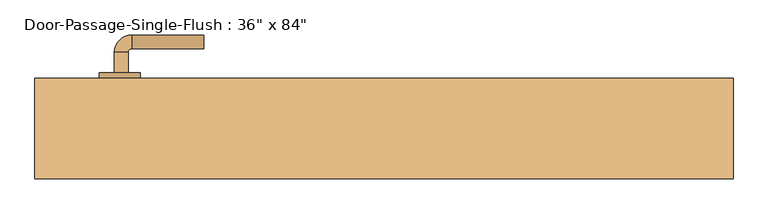
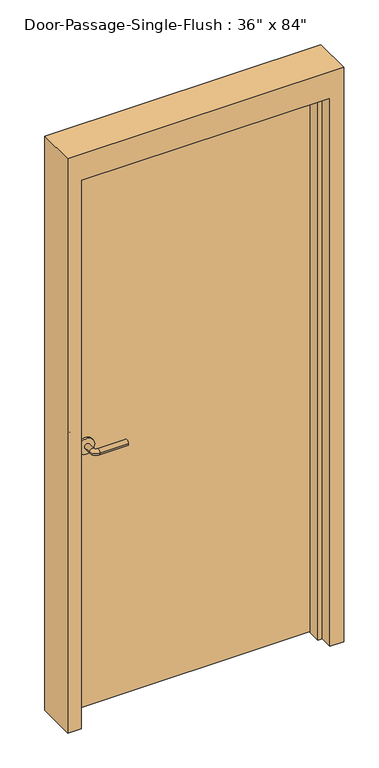
"""IFC4 building model written with IfcOpenShell, lengths in millimetres: door geometry."""

from ifc_helpers import new_model, si_unit, point, frame, frame_2d, origin, origin_with_axes, place, context, project, spatial, polyline, circle_curve, ellipse_curve, trimmed, segment, composite_curve, outline, extrude, faceted_brep, source, transform, mapped, element, save
from ifc_brep_helpers import plane_surface, cylinder_surface, revolved_surface, advanced_brep


def door_9ff278b0(model_context):
    return source(origin(), model_context, "Body", "SolidModel", [
        advanced_brep(
        [(-392.190625, 42.8, 1016.0), (-372.190625, 42.8, 1016.0), (-372.190625, 12.8, 1016.0), (-392.190625, 12.8, 1016.0), (-367.190625, 7.8, 1016.0), (-367.190625, -12.2, 1016.0), (-262.190625, -12.2, 1016.0), (-262.190625, 7.8, 1016.0)],
        [
            (0, 1, circle_curve(frame((-382.190625, 42.8, 1016.0), z_axis=(0.0, 1.0, 0.0), x_axis=(1.0, 0.0, 0.0)), 10.0)),
            (1, 0, circle_curve(frame((-382.190625, 42.8, 1016.0), z_axis=(0.0, 1.0, 0.0), x_axis=(1.0, 0.0, 0.0)), 10.0)),
            (1, 2),
            (2, 3, circle_curve(frame((-382.190625, 12.8, 1016.0), z_axis=(0.0, 1.0, 0.0), x_axis=(1.0, 0.0, 0.0)), 10.0)),
            (3, 0),
            (3, 2, circle_curve(frame((-382.190625, 12.8, 1016.0), z_axis=(0.0, 1.0, 0.0), x_axis=(1.0, 0.0, 0.0)), 10.0)),
            (4, 5, circle_curve(frame((-367.190625, -2.2, 1016.0), z_axis=(-1.0, 0.0, 0.0), x_axis=(0.0, 1.0, 0.0)), 10.0)),
            (5, 3, circle_curve(frame((-367.190625, 12.8, 1016.0), z_axis=(0.0, 0.0, -1.0), x_axis=(-1.0, 0.0, 0.0)), 25.0)),
            (2, 4, circle_curve(frame((-367.190625, 12.8, 1016.0), z_axis=(0.0, 0.0, 1.0), x_axis=(-1.0, 0.0, 0.0)), 5.0)),
            (5, 4, circle_curve(frame((-367.190625, -2.2, 1016.0), z_axis=(-1.0, 0.0, 0.0), x_axis=(0.0, 1.0, 0.0)), 10.0)),
            (6, 7, circle_curve(frame((-262.190625, -2.2, 1016.0), z_axis=(1.0, 0.0, 0.0), x_axis=(0.0, 1.0, 0.0)), 10.0)),
            (7, 6, circle_curve(frame((-262.190625, -2.2, 1016.0), z_axis=(1.0, 0.0, 0.0), x_axis=(0.0, 1.0, 0.0)), 10.0)),
            (4, 7),
            (6, 5),
        ],
        [
            plane_surface(frame((-382.190625, 42.8, 1016.0), z_axis=(0.0, 1.0, 0.0), x_axis=(0.0, 0.0, 1.0))),
            cylinder_surface(frame((-382.190625, 42.8, 1016.0), z_axis=(0.0, 1.0, 0.0), x_axis=(1.0, 0.0, 0.0)), 10.0),
            revolved_surface(trimmed(ellipse_curve(frame((-382.190625, 12.8, 1016.0), z_axis=(0.0, -1.0, 0.0), x_axis=(1.0, 0.0, 0.0)), 10.0, 10.0), [point((-392.190625, 12.8, 1016.0))], [point((-372.190625, 12.8, 1016.0))], True, "CARTESIAN"), (-367.190625, 12.8, 1016.0), (0.0, 0.0, -1.0)),
            revolved_surface(trimmed(ellipse_curve(frame((-382.190625, 12.8, 1016.0), z_axis=(0.0, -1.0, 0.0), x_axis=(1.0, 0.0, 0.0)), 10.0, 10.0), [point((-372.190625, 12.8, 1016.0))], [point((-392.190625, 12.8, 1016.0))], True, "CARTESIAN"), (-367.190625, 12.8, 1016.0), (0.0, 0.0, -1.0)),
            plane_surface(frame((-262.190625, -2.2, 1016.0), z_axis=(1.0, 0.0, 0.0), x_axis=(0.0, 0.0, 1.0))),
            cylinder_surface(frame((-367.190625, -2.2, 1016.0), z_axis=(-1.0, 0.0, 0.0), x_axis=(0.0, 1.0, 0.0)), 10.0),
        ],
        [
            (0, [[1, 2]]),
            (1, [[3, 4, 5, -2]]),
            (1, [[-5, 6, -3, -1]]),
            (2, [[7, 8, -4, 9]]),
            (3, [[10, -9, -6, -8]]),
            (4, [[11, 12]]),
            (5, [[13, -11, 14, -7]]),
            (5, [[-14, -12, -13, -10]]),
        ],
    ),
        extrude(outline(composite_curve([segment(trimmed(circle_curve(frame_2d((1016.0, -384.690625)), 30.0), [point((1016.0, -414.690625))], [point((1016.0, -354.690625))], False, "CARTESIAN"), True, "CONTINUOUS"), segment(trimmed(circle_curve(frame_2d((1016.0, -384.690625)), 30.0), [point((1016.0, -354.690625))], [point((1016.0, -414.690625))], False, "CARTESIAN"), True, "CONTINUOUS")], self_intersect=False)), frame((0.0, 42.8, 0.0), z_axis=(0.0, 1.0, 0.0), x_axis=(0.0, 0.0, 1.0)), (0.0, 0.0, 1.0), 8.0),
        advanced_brep(
        [(-392.190625, 103.25, 1016.0), (-372.190625, 103.25, 1016.0), (-392.190625, 133.25, 1016.0), (-372.190625, 133.25, 1016.0), (-367.190625, 138.25, 1016.0), (-367.190625, 158.25, 1016.0), (-262.190625, 158.25, 1016.0), (-262.190625, 138.25, 1016.0)],
        [
            (0, 1, circle_curve(frame((-382.190625, 103.25, 1016.0), z_axis=(0.0, -1.0, 0.0), x_axis=(1.0, 0.0, 0.0)), 10.0)),
            (1, 0, circle_curve(frame((-382.190625, 103.25, 1016.0), z_axis=(0.0, -1.0, 0.0), x_axis=(1.0, 0.0, 0.0)), 10.0)),
            (0, 2),
            (2, 3, circle_curve(frame((-382.190625, 133.25, 1016.0), z_axis=(0.0, -1.0, 0.0), x_axis=(1.0, 0.0, 0.0)), 10.0)),
            (3, 1),
            (3, 2, circle_curve(frame((-382.190625, 133.25, 1016.0), z_axis=(0.0, -1.0, 0.0), x_axis=(1.0, 0.0, 0.0)), 10.0)),
            (4, 3, circle_curve(frame((-367.190625, 133.25, 1016.0), z_axis=(0.0, 0.0, 1.0), x_axis=(-1.0, 0.0, 0.0)), 5.0)),
            (2, 5, circle_curve(frame((-367.190625, 133.25, 1016.0), z_axis=(0.0, 0.0, -1.0), x_axis=(-1.0, 0.0, 0.0)), 25.0)),
            (5, 4, circle_curve(frame((-367.190625, 148.25, 1016.0), z_axis=(-1.0, 0.0, 0.0), x_axis=(0.0, -1.0, 0.0)), 10.0)),
            (4, 5, circle_curve(frame((-367.190625, 148.25, 1016.0), z_axis=(-1.0, 0.0, 0.0), x_axis=(0.0, -1.0, 0.0)), 10.0)),
            (6, 7, circle_curve(frame((-262.190625, 148.25, 1016.0), z_axis=(1.0, 0.0, 0.0), x_axis=(0.0, -1.0, 0.0)), 10.0)),
            (7, 6, circle_curve(frame((-262.190625, 148.25, 1016.0), z_axis=(1.0, 0.0, 0.0), x_axis=(0.0, -1.0, 0.0)), 10.0)),
            (5, 6),
            (7, 4),
        ],
        [
            plane_surface(frame((-382.190625, 103.25, 1016.0), z_axis=(0.0, -1.0, 0.0), x_axis=(0.0, 0.0, 1.0))),
            cylinder_surface(frame((-382.190625, 103.25, 1016.0), z_axis=(0.0, -1.0, 0.0), x_axis=(1.0, 0.0, 0.0)), 10.0),
            revolved_surface(trimmed(ellipse_curve(frame((-382.190625, 133.25, 1016.0), z_axis=(0.0, -1.0, 0.0), x_axis=(1.0, 0.0, 0.0)), 10.0, 10.0), [point((-392.190625, 133.25, 1016.0))], [point((-372.190625, 133.25, 1016.0))], True, "CARTESIAN"), (-367.190625, 133.25, 1016.0), (0.0, 0.0, -1.0)),
            revolved_surface(trimmed(ellipse_curve(frame((-382.190625, 133.25, 1016.0), z_axis=(0.0, -1.0, 0.0), x_axis=(1.0, 0.0, 0.0)), 10.0, 10.0), [point((-372.190625, 133.25, 1016.0))], [point((-392.190625, 133.25, 1016.0))], True, "CARTESIAN"), (-367.190625, 133.25, 1016.0), (0.0, 0.0, -1.0)),
            plane_surface(frame((-262.190625, 148.25, 1016.0), z_axis=(1.0, 0.0, 0.0), x_axis=(0.0, 0.0, 1.0))),
            cylinder_surface(frame((-367.190625, 148.25, 1016.0), z_axis=(-1.0, 0.0, 0.0), x_axis=(0.0, -1.0, 0.0)), 10.0),
        ],
        [
            (0, [[1, 2]]),
            (1, [[-1, 3, 4, 5]]),
            (1, [[-2, -5, 6, -3]]),
            (2, [[7, -4, 8, 9]]),
            (3, [[-8, -6, -7, 10]]),
            (4, [[11, 12]]),
            (5, [[-9, 13, -12, 14]]),
            (5, [[-10, -14, -11, -13]]),
        ],
    ),
        extrude(outline(composite_curve([segment(trimmed(circle_curve(frame_2d((1016.0, -384.690625)), 30.0), [point((1016.0, -414.690625))], [point((1016.0, -354.690625))], False, "CARTESIAN"), True, "CONTINUOUS"), segment(trimmed(circle_curve(frame_2d((1016.0, -384.690625)), 30.0), [point((1016.0, -354.690625))], [point((1016.0, -414.690625))], False, "CARTESIAN"), True, "CONTINUOUS")], self_intersect=False)), frame((0.0, 95.25, 0.0), z_axis=(0.0, 1.0, 0.0), x_axis=(0.0, 0.0, 1.0)), (0.0, 0.0, 1.0), 8.0),
        faceted_brep([(457.2, 46.0375, 0.0), (457.2, 95.25, 0.0), (508.0, 95.25, 0.0), (508.0, -50.8, 0.0), (457.2, -50.8, 0.0), (457.2, -1.5875, 0.0), (441.325, -1.5875, 0.0), (441.325, 46.0375, 0.0), (457.2, 46.0375, 2133.6), (457.2, 95.25, 2133.6), (-457.2, 95.25, 2133.6), (-457.2, 95.25, 0.0), (-508.0, 95.25, 0.0), (-508.0, 95.25, 2235.2), (508.0, 95.25, 2235.2), (508.0, -50.8, 2235.2), (-508.0, -50.8, 2235.2), (-508.0, -50.8, 0.0), (-457.2, -50.8, 0.0), (-457.2, -50.8, 2133.6), (457.2, -50.8, 2133.6), (457.2, -1.5875, 2133.6), (-457.2, -1.5875, 2133.6), (-457.2, -1.5875, 0.0), (-441.325, -1.5875, 0.0), (-441.325, -1.5875, 2117.725), (441.325, -1.5875, 2117.725), (441.325, 46.0375, 2117.725), (-441.325, 46.0375, 2117.725), (-441.325, 46.0375, 0.0), (-457.2, 46.0375, 0.0), (-457.2, 46.0375, 2133.6)], [[[0, 1, 2, 3, 4, 5, 6, 7]], [[1, 0, 8, 9]], [[2, 1, 9, 10, 11, 12, 13, 14]], [[3, 2, 14, 15]], [[4, 3, 15, 16, 17, 18, 19, 20]], [[5, 4, 20, 21]], [[6, 5, 21, 22, 23, 24, 25, 26]], [[7, 6, 26, 27]], [[0, 7, 27, 28, 29, 30, 31, 8]], [[9, 8, 31, 10]], [[20, 19, 22, 21]], [[26, 25, 28, 27]], [[12, 11, 30, 29, 24, 23, 18, 17]], [[11, 10, 31, 30]], [[13, 12, 17, 16]], [[19, 18, 23, 22]], [[25, 24, 29, 28]], [[15, 14, 13, 16]]]),
        extrude(outline(polyline([(457.2, 50.8), (-457.2, 50.8), (-457.2, 95.25), (457.2, 95.25), (457.2, 50.8)])), origin_with_axes(), (0.0, 0.0, 1.0), 2133.6),
    ])


if __name__ == "__main__":
    model = new_model("IFC4")
    model_context = context("Model", 3, world=origin())
    ifc_project = project(units=[si_unit("LENGTHUNIT", "METRE", prefix="MILLI")], contexts=[model_context])
    site = spatial("IfcSite", under=ifc_project)
    building = spatial("IfcBuilding", under=site)
    placement = place(None, origin())
    door_shape = door_9ff278b0(model_context)
    element("IfcDoor", 1, ObjectType="Door-Passage-Single-Flush : 36\" x 84\"", at=placement, inside=building, context=model_context, shape_type="MappedRepresentation", body=[
        mapped(door_shape, transform((0.0, 0.0, 0.0), x_axis=(1.0, 0.0, 0.0), y_axis=(0.0, 1.0, 0.0), z_axis=(0.0, 0.0, 1.0))),
    ])
    save(model, "model.ifc")

# Revit data of these elements
# Type "Door-Passage-Single-Flush : 36\" x 84\""
#   Type Mark = "11"
#   Assembly Code = "B2030200"
#   Analytic Construction = "Wooden"
#   Thickness = 0' - 1 3/4"
#   Thermal Resistance (R) = 2.5876 (h·ft²·°F)/BTU
#   Swing Angle [instance default] = 90.00°
#   Strike Height = 3' - 4"
#   Rough Width [instance default] = 3' - 4"
#   Rough Height [instance default] = 7' - 4"
#   MF Opening Height [instance default] = 0' - 4"
#   MF Opening Width [instance default] = 0' - 4"
#   Inset Calculate [instance default] = 0' - 4"
#   Masonry Inset [instance default] = 0' - 1"
#   Height = 7' - 0"
#   Width = 3' - 0"
#   Heat Transfer Coefficient (U) = 0.3865 BTU/(h·ft²·°F)
#   Masonry Frame Depth = 0' - 5 3/4"
#   Masonry Frame [instance default] = yes
#   Function = 1
#   Dry Wall Frame [instance default] = no
#   Define Thermal Properties by = 1
#   Panel Material = Wood - Birch
#   Frame Material = Metal - Paint Finish - Grey
#   Door Handle Material = Aluminum
#   Visual Light Transmittance = 0
#   Solar Heat Gain Coefficient = 0
#   Wall Closure = (empty or 0)
# Element 1 (IfcDoor, "Door-Passage-Single-Flush : 36\" x 84\"")
#   Materials on its faces: "Aluminum", "Metal - Paint Finish - Grey", "Wood - Birch"
# Materials
#   "Wood - Birch": class "Wood", colour RGB 173 132 96, transparency 0, Cost = 0
#   "Metal - Paint Finish - Grey": class "Paint", colour RGB 178 178 178, transparency 0, Cost = 0
#   "Aluminum": class "Metal", colour RGB 244 245 246, transparency 0, Description = "Aluminum 6061", Cost = 0
